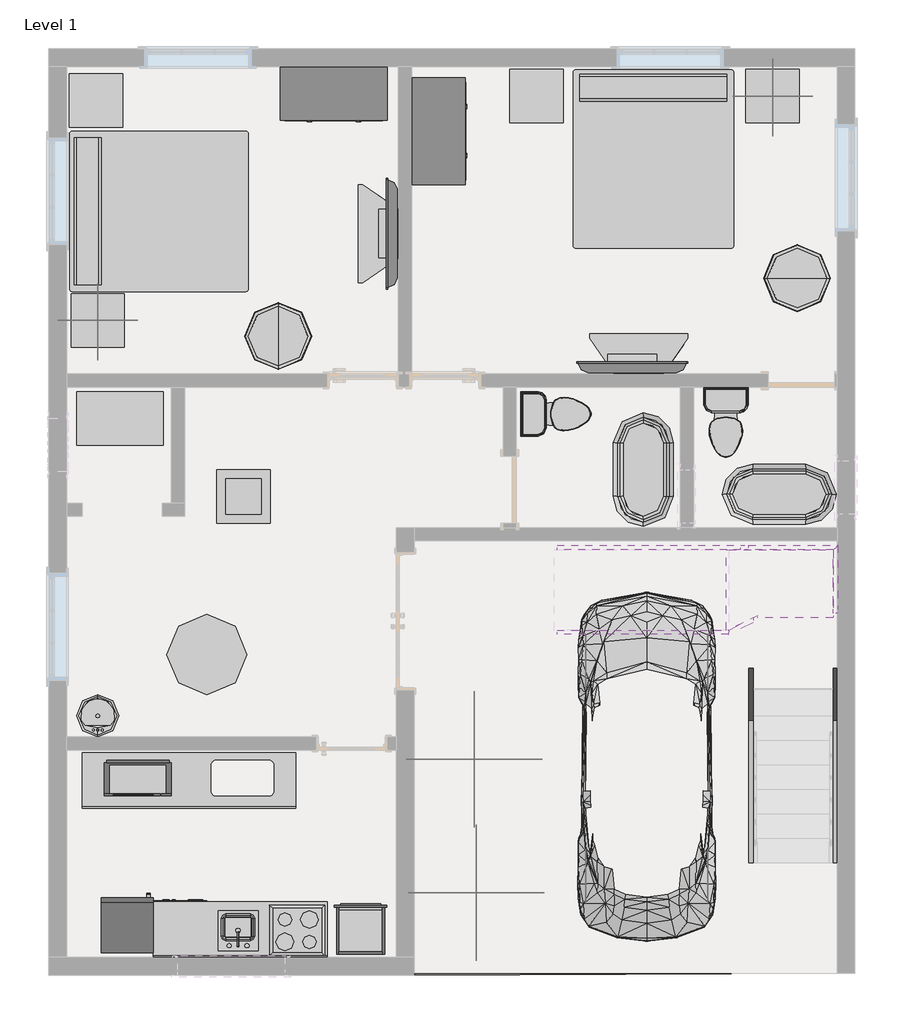
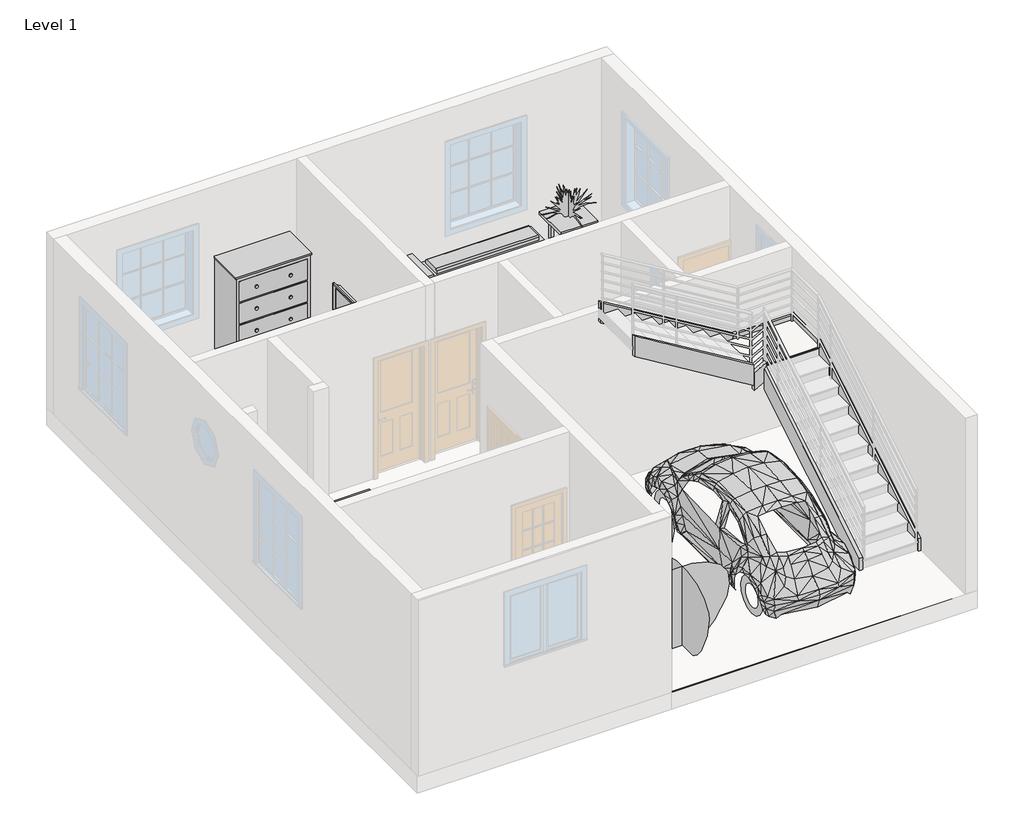
# One storey, part 5 of 5: 19 furniture elements, 8 proxies, 7 members, 6 flow terminals, 4 geographic elements, 1 slab.
"""IFC4 building model written with IfcOpenShell, lengths in millimetres."""

from ifc_helpers import new_model, si_unit, frame, origin, place, context, project, spatial, polyline, outline, extrude, faceted_brep, triangles, transform, mapped, element, save
from components import proxy_a6faaae8, proxy_45b28599, kitchenette_medium_kitchenette_medium_844211aa, proxy_8a8d5ab2, proxy_8b8c2dc4, rpc_beetle_rpc_beetle_3ce7ba48, proxy_c523a7b7, flow_terminal_871c2e40, flow_terminal_d49f872f, toilet_domestic_3d_toilet_domestic_3d_f7549cf7, toilet_domestic_3d_toilet_domestic_3d_183bbd19, flow_terminal_93af9e75, furniture_a8794613, furniture_22cae41e, furniture_c6510c7c, furniture_9fa109b2, furniture_fdf74506, tv_stand_tv_stand_6ce107e5, furniture_b5c51a22, furniture_905aceb5, furniture_5bc9ed15, furniture_d861f60e, furniture_ebfaaaa6, rpc_plant_tropical_agave_1_5_93a2a214, geographic_element_ca6e1e19, non_monolithic_landing_e53bceee

model = new_model("IFC4")

# Units and contexts
model_context = context("Model", 3, world=origin())
ifc_project = project(units=[si_unit("LENGTHUNIT", "METRE", prefix="MILLI")], contexts=[model_context])

# Site, building, storey
site = spatial("IfcSite", under=ifc_project)
building = spatial("IfcBuilding", under=site)
storey = spatial("IfcBuildingStorey", under=building, Name="Level 1", Elevation=0.0)

# Proxies
placement = place(None, origin())
element("IfcBuildingElementProxy", 1, Name="Building Element Proxy", at=placement, inside=storey, context=model_context, shape_type="Tessellation", body=[
    triangles([(-5848.5895203, 6522.5448944, 0.0), (-1156.9729843, 6792.048793, 0.0), (-1156.9729843, 2097.9200558, 0.0), (-5982.9731781, 2072.5200073, 0.0), (-5919.2578812, 6787.1200241, 0.0), (-5945.4754669, 6669.6818436, 0.0), (-5982.9731781, 7000.1198135, 0.0), (-1156.9729843, 6947.7020828, 0.0)], [[4, 6, 7], [5, 6, 1], [7, 5, 8], [5, 7, 6], [6, 4, 1], [1, 3, 2], [3, 1, 4], [2, 8, 1], [1, 8, 5]], closed=False),
])
proxy_shape = proxy_a6faaae8(model_context)
element("IfcBuildingElementProxy", 2, Name="Cook Top-4 Unit2 : 22\" x 20\"", ObjectType="Cook Top-4 Unit2 : 22\" x 20\"", at=placement, inside=storey, context=model_context, shape_type="MappedRepresentation", body=[
    mapped(proxy_shape, transform((-7316.4730118, 2580.5200123, 0.0), x_axis=(-1.0000000000000004, 0.0, 0.0), y_axis=(0.0, -1.0000000000000004, 0.0), z_axis=(0.0, 0.0, 1.0))),
])
proxy_2_shape = proxy_45b28599(model_context)
element("IfcBuildingElementProxy", 3, Name="Dishwasher : 24\" x 24\" x 34\"", ObjectType="Dishwasher : 24\" x 24\" x 34\"", at=placement, inside=storey, context=model_context, shape_type="MappedRepresentation", body=[
    mapped(proxy_2_shape, transform((-8267.6555433, 2872.3695771, 0.0), x_axis=(-1.0000000000000004, 0.0, 0.0), y_axis=(0.0, -1.0000000000000004, 0.0), z_axis=(0.0, 0.0, 1.0))),
])
kitchenette_medium_kitchenette_medium_shape = kitchenette_medium_kitchenette_medium_844211aa(model_context)
element("IfcBuildingElementProxy", 4, Name="Kitchenette - Medium : Kitchenette - Medium", ObjectType="Kitchenette - Medium : Kitchenette - Medium", at=placement, inside=storey, context=model_context, shape_type="MappedRepresentation", body=[
    mapped(kitchenette_medium_kitchenette_medium_shape, transform((-7640.6353069, 2275.7200123, 0.0), x_axis=(-1.0000000000000004, 0.0, 0.0), y_axis=(0.0, -1.0000000000000004, 0.0), z_axis=(0.0, 0.0, 1.0))),
])
proxy_3_shape = proxy_8a8d5ab2(model_context)
element("IfcBuildingElementProxy", 5, Name="Microwave : 30\" x 16\" x 18\"", ObjectType="Microwave : 30\" x 16\" x 18\"", at=placement, inside=storey, context=model_context, shape_type="MappedRepresentation", body=[
    mapped(proxy_3_shape, transform((-9632.8658891, 4673.5005181, 0.0), x_axis=(1.0000000000000007, 0.0, 0.0), y_axis=(0.0, 1.0000000000000007, 0.0), z_axis=(0.0, 0.0, 1.0))),
])
proxy_4_shape = proxy_8b8c2dc4(model_context)
element("IfcBuildingElementProxy", 6, Name="Oven Double-Built-in : 21 1/2\" x 39 1/4\" x 21\"", ObjectType="Oven Double-Built-in : 21 1/2\" x 39 1/4\" x 21\"", at=placement, inside=storey, context=model_context, shape_type="MappedRepresentation", body=[
    mapped(proxy_4_shape, transform((-6627.7479391, 2721.5858712, 0.0), x_axis=(-1.0000000000000004, 0.0, 0.0), y_axis=(0.0, -1.0000000000000004, 0.0), z_axis=(0.0, 0.0, 1.0))),
])
rpc_beetle_rpc_beetle_shape = rpc_beetle_rpc_beetle_3ce7ba48(model_context)
element("IfcBuildingElementProxy", 7, Name="RPC Beetle : RPC Beetle", ObjectType="RPC Beetle : RPC Beetle", at=placement, inside=storey, context=model_context, shape_type="MappedRepresentation", body=[
    mapped(rpc_beetle_rpc_beetle_shape, transform((-3328.6730118, 3215.5200123, 0.0), x_axis=(1.0, 0.0, 0.0), y_axis=(0.0, 1.0, 0.0), z_axis=(0.0, 0.0, 1.0))),
])
proxy_5_shape = proxy_c523a7b7(model_context)
element("IfcBuildingElementProxy", 8, Name="Refrigerator : 24\" x 25\" LH", ObjectType="Refrigerator : 24\" x 25\" LH", at=placement, inside=storey, context=model_context, shape_type="MappedRepresentation", body=[
    mapped(proxy_5_shape, transform((-9253.2230118, 2626.1689838, 0.0), x_axis=(-1.0000000000000004, 0.0, 0.0), y_axis=(0.0, -1.0000000000000004, 0.0), z_axis=(0.0, 0.0, 1.0))),
])

# Flow terminals
flow_terminal_shape = flow_terminal_871c2e40(model_context)
element("IfcFlowTerminal", 9, ObjectType="Sink Kitchen-Island : 18\" x 18\"", at=placement, inside=storey, context=model_context, shape_type="MappedRepresentation", body=[
    mapped(flow_terminal_shape, transform((-7973.8837712, 2582.8654134, -14.4), x_axis=(-1.0000000000000004, 0.0, 0.0), y_axis=(0.0, -1.0000000000000004, 0.0), z_axis=(0.0, 0.0, 1.0))),
])
flow_terminal_2_shape = flow_terminal_d49f872f(model_context)
element("IfcFlowTerminal", 10, ObjectType="Sink Vanity-Round : 19\" x 19\"", at=placement, inside=storey, context=model_context, shape_type="MappedRepresentation", body=[
    mapped(flow_terminal_2_shape, transform((-9493.1212712, 5116.6266447, 304.8), x_axis=(-1.0000000000000004, 0.0, 0.0), y_axis=(0.0, -1.0000000000000004, 0.0), z_axis=(0.0, 0.0, 1.0))),
])
toilet_domestic_3d_toilet_domestic_3d_shape = toilet_domestic_3d_toilet_domestic_3d_f7549cf7(model_context)
toilet_domestic_3d_toilet_domestic_3d_2_shape = toilet_domestic_3d_toilet_domestic_3d_183bbd19(model_context)
element("IfcFlowTerminal", 11, ObjectType="Toilet-Domestic-3D : Toilet-Domestic-3D", at=placement, inside=storey, context=model_context, shape_type="MappedRepresentation", body=[
    mapped(toilet_domestic_3d_toilet_domestic_3d_shape, transform((-2426.9730118, 8283.4239849, 0.0), x_axis=(1.0000000000000007, 0.0, 0.0), y_axis=(0.0, 1.0000000000000007, 0.0), z_axis=(0.0, 0.0, 1.0))),
    mapped(toilet_domestic_3d_toilet_domestic_3d_2_shape, transform((-2426.9730118, 8283.4239849, 0.0), x_axis=(1.0000000000000007, 0.0, 0.0), y_axis=(0.0, 1.0000000000000007, 0.0), z_axis=(0.0, 0.0, 1.0))),
])
element("IfcFlowTerminal", 12, ObjectType="Toilet-Domestic-3D : Toilet-Domestic-3D", at=placement, inside=storey, context=model_context, shape_type="MappedRepresentation", body=[
    mapped(toilet_domestic_3d_toilet_domestic_3d_shape, transform((-4269.0769845, 8473.3200123, 0.0), x_axis=(0.0, 1.0000000000000002, 0.0), y_axis=(-1.0000000000000002, 0.0, 0.0), z_axis=(0.0, 0.0, 1.0))),
    mapped(toilet_domestic_3d_toilet_domestic_3d_2_shape, transform((-4269.0769845, 8473.3200123, 0.0), x_axis=(0.0, 1.0000000000000002, 0.0), y_axis=(-1.0000000000000002, 0.0, 0.0), z_axis=(0.0, 0.0, 1.0))),
])
flow_terminal_3_shape = flow_terminal_93af9e75(model_context)
element("IfcFlowTerminal", 13, ObjectType="Tub-Free Standing-3D : 30\" x 60\"", at=placement, inside=storey, context=model_context, shape_type="MappedRepresentation", body=[
    mapped(flow_terminal_3_shape, transform((-1817.3730118, 7558.9200123, 0.0), x_axis=(0.0, -1.0000000000000002, 0.0), y_axis=(1.0000000000000002, 0.0, 0.0), z_axis=(0.0, 0.0, 1.0))),
])
element("IfcFlowTerminal", 14, ObjectType="Tub-Free Standing-3D : 30\" x 60\"", at=placement, inside=storey, context=model_context, shape_type="MappedRepresentation", body=[
    mapped(flow_terminal_3_shape, transform((-3366.7730118, 7838.3200123, 0.0), x_axis=(-1.0000000000000004, 0.0, 0.0), y_axis=(0.0, -1.0000000000000004, 0.0), z_axis=(0.0, 0.0, 1.0))),
])

# Furniture
furniture_shape = furniture_a8794613(model_context)
element("IfcFurniture", 15, ObjectType="Bed-Standard.0001 : King 78\" x 80\"", at=placement, inside=storey, context=model_context, shape_type="MappedRepresentation", body=[
    mapped(furniture_shape, transform((-8936.8680938, 10513.2314877, 0.0), x_axis=(0.0, 1.0000000000000002, 0.0), y_axis=(-1.0000000000000002, 0.0, 0.0), z_axis=(0.0, 0.0, 1.0))),
])
element("IfcFurniture", 16, ObjectType="Bed-Standard.0001 : King 78\" x 80\"", at=placement, inside=storey, context=model_context, shape_type="MappedRepresentation", body=[
    mapped(furniture_shape, transform((-3523.9615364, 11427.2150942, 0.0), x_axis=(1.0, 0.0, 0.0), y_axis=(0.0, 1.0, 0.0), z_axis=(0.0, 0.0, 1.0))),
])
furniture_2_shape = furniture_22cae41e(model_context)
element("IfcFurniture", 17, ObjectType="Counter Top w Sink Hole : 24\" Depth", at=placement, inside=storey, context=model_context, shape_type="MappedRepresentation", body=[
    mapped(furniture_2_shape, transform((-8529.6353069, 3977.5200123, 0.0), x_axis=(-1.0000000000000002, 0.0, 0.0), y_axis=(0.0, -1.0000000000000002, 0.0), z_axis=(0.0, 0.0, 1.0))),
])
furniture_3_shape = furniture_c6510c7c(model_context)
element("IfcFurniture", 18, ObjectType="Counter Top w Sink Hole : 24\" Depth", at=placement, inside=storey, context=model_context, shape_type="MappedRepresentation", body=[
    mapped(furniture_3_shape, transform((-8174.0353069, 2275.7200123, -14.4), x_axis=(-1.0000000000000004, 0.0, 0.0), y_axis=(0.0, -1.0000000000000004, 0.0), z_axis=(0.0, 0.0, 1.0))),
])
furniture_4_shape = furniture_9fa109b2(model_context)
element("IfcFurniture", 19, ObjectType="Dresser : 48\" x 72\" x 24\"", at=placement, inside=storey, context=model_context, shape_type="MappedRepresentation", body=[
    mapped(furniture_4_shape, transform((-6628.179752, 12494.0829664, 0.0), x_axis=(1.0, 0.0, 0.0), y_axis=(0.0, 1.0, 0.0), z_axis=(0.0, 0.0, 1.0))),
])
element("IfcFurniture", 20, ObjectType="Dresser : 48\" x 72\" x 24\"", at=placement, inside=storey, context=model_context, shape_type="MappedRepresentation", body=[
    mapped(furniture_4_shape, transform((-6066.7359659, 11968.3132721, 0.0), x_axis=(0.0, 1.0000000000000002, 0.0), y_axis=(-1.0000000000000002, 0.0, 0.0), z_axis=(0.0, 0.0, 1.0))),
])
furniture_5_shape = furniture_fdf74506(model_context)
element("IfcFurniture", 21, ObjectType="TV - Flat Screen : 50\"", at=placement, inside=storey, context=model_context, shape_type="MappedRepresentation", body=[
    mapped(furniture_5_shape, transform((-6232.0116355, 10526.7754981, 914.4), x_axis=(0.0, -1.0, 0.0), y_axis=(1.0, 0.0, 0.0), z_axis=(0.0, 0.0, 1.0))),
])
element("IfcFurniture", 22, ObjectType="TV - Flat Screen : 50\"", at=placement, inside=storey, context=model_context, shape_type="MappedRepresentation", body=[
    mapped(furniture_5_shape, transform((-3497.717526, 9001.7586359, 914.4), x_axis=(-1.0000000000000004, 0.0, 0.0), y_axis=(0.0, -1.0000000000000004, 0.0), z_axis=(0.0, 0.0, 1.0))),
])
tv_stand_tv_stand_shape = tv_stand_tv_stand_6ce107e5(model_context)
element("IfcFurniture", 23, ObjectType="TV Stand : TV Stand", at=placement, inside=storey, context=model_context, shape_type="MappedRepresentation", body=[
    mapped(tv_stand_tv_stand_shape, transform((-6160.7730118, 10655.9080143, 0.0), x_axis=(0.0, -1.0000000000000002, 0.0), y_axis=(1.0000000000000002, 0.0, 0.0), z_axis=(0.0, 0.0, 1.0))),
])
element("IfcFurniture", 24, ObjectType="TV Stand : TV Stand", at=placement, inside=storey, context=model_context, shape_type="MappedRepresentation", body=[
    mapped(tv_stand_tv_stand_shape, transform((-3292.3850097, 8930.5200123, 0.0), x_axis=(-1.0000000000000002, 0.0, 0.0), y_axis=(0.0, -1.0000000000000002, 0.0), z_axis=(0.0, 0.0, 1.0))),
])
furniture_6_shape = furniture_b5c51a22(model_context)
element("IfcFurniture", 25, ObjectType="Table-Coffee : 24\" x 24\" x 24\"", at=placement, inside=storey, context=model_context, shape_type="MappedRepresentation", body=[
    mapped(furniture_6_shape, transform((-7944.3387785, 7438.3089345, 0.0), x_axis=(1.0, 0.0, 0.0), y_axis=(0.0, 1.0, 0.0), z_axis=(0.0, 0.0, 1.0))),
])
furniture_7_shape = furniture_905aceb5(model_context)
element("IfcFurniture", 26, ObjectType="Table-Dining Round w Chairs : 36\" Diameter", at=placement, inside=storey, context=model_context, shape_type="MappedRepresentation", body=[
    mapped(furniture_7_shape, transform((-8448.854979, 5914.9987008, 0.0), x_axis=(1.0, 0.0, 0.0), y_axis=(0.0, 1.0, 0.0), z_axis=(0.0, 0.0, 1.0))),
])
furniture_8_shape = furniture_5bc9ed15(model_context)
element("IfcFurniture", 27, ObjectType="Table-Night Stand : 24\" x 24\" x 30\"", at=placement, inside=storey, context=model_context, shape_type="MappedRepresentation", body=[
    mapped(furniture_8_shape, transform((-9898.3066421, 9235.3200123, 0.0), x_axis=(1.0, 0.0, 0.0), y_axis=(0.0, 1.0, 0.0), z_axis=(0.0, 0.0, 1.0))),
])
element("IfcFurniture", 28, ObjectType="Table-Night Stand : 24\" x 24\" x 30\"", at=placement, inside=storey, context=model_context, shape_type="MappedRepresentation", body=[
    mapped(furniture_8_shape, transform((-9917.3566421, 11743.5700123, 0.0), x_axis=(1.0, 0.0, 0.0), y_axis=(0.0, 1.0, 0.0), z_axis=(0.0, 0.0, 1.0))),
])
element("IfcFurniture", 29, ObjectType="Table-Night Stand : 24\" x 24\" x 30\"", at=placement, inside=storey, context=model_context, shape_type="MappedRepresentation", body=[
    mapped(furniture_8_shape, transform((-2202.1066421, 11794.3700123, 0.0), x_axis=(1.0, 0.0, 0.0), y_axis=(0.0, 1.0, 0.0), z_axis=(0.0, 0.0, 1.0))),
])
element("IfcFurniture", 30, ObjectType="Table-Night Stand : 24\" x 24\" x 30\"", at=placement, inside=storey, context=model_context, shape_type="MappedRepresentation", body=[
    mapped(furniture_8_shape, transform((-4894.5066421, 11794.3700123, 0.0), x_axis=(1.0, 0.0, 0.0), y_axis=(0.0, 1.0, 0.0), z_axis=(0.0, 0.0, 1.0))),
])
furniture_9_shape = furniture_d861f60e(model_context)
element("IfcFurniture", 31, ObjectType="Table-Rectangular : 72\" x 30\"", at=placement, inside=storey, context=model_context, shape_type="MappedRepresentation", body=[
    mapped(furniture_9_shape, transform((-9335.7730118, 8422.5200123, 0.0), x_axis=(1.0, 0.0, 0.0), y_axis=(0.0, 1.0, 0.0), z_axis=(0.0, 0.0, 1.0))),
])
furniture_10_shape = furniture_ebfaaaa6(model_context)
element("IfcFurniture", 32, ObjectType="Table-Round : 36\" Diameter", at=placement, inside=storey, context=model_context, shape_type="MappedRepresentation", body=[
    mapped(furniture_10_shape, transform((-7532.3730118, 9362.3200123, 0.0), x_axis=(0.0, 1.0000000000000002, 0.0), y_axis=(-1.0000000000000002, 0.0, 0.0), z_axis=(0.0, 0.0, 1.0))),
])
element("IfcFurniture", 33, ObjectType="Table-Round : 36\" Diameter", at=placement, inside=storey, context=model_context, shape_type="MappedRepresentation", body=[
    mapped(furniture_10_shape, transform((-1614.1730118, 10022.7200123, 0.0), x_axis=(1.0, 0.0, 0.0), y_axis=(0.0, 1.0, 0.0), z_axis=(0.0, 0.0, 1.0))),
])

# Geographic elements
rpc_plant_tropical_agave_1_5_shape = rpc_plant_tropical_agave_1_5_93a2a214(model_context)
element("IfcGeographicElement", 34, ObjectType="RPC Plant - Tropical : Agave - 1.5'", at=placement, inside=storey, context=model_context, shape_type="MappedRepresentation", body=[
    mapped(rpc_plant_tropical_agave_1_5_shape, transform((-9589.7730118, 9540.1200123, 762.0), x_axis=(1.0, 0.0, 0.0), y_axis=(0.0, 1.0, 0.0), z_axis=(0.0, 0.0, 1.0))),
])
element("IfcGeographicElement", 35, ObjectType="RPC Plant - Tropical : Agave - 1.5'", at=placement, inside=storey, context=model_context, shape_type="MappedRepresentation", body=[
    mapped(rpc_plant_tropical_agave_1_5_shape, transform((-1893.5730118, 12099.1700123, 762.0), x_axis=(1.0, 0.0, 0.0), y_axis=(0.0, 1.0, 0.0), z_axis=(0.0, 0.0, 1.0))),
])
geographic_element_shape = geographic_element_ca6e1e19(model_context)
element("IfcGeographicElement", 36, ObjectType="RPC Shrub : Burning Bush 4'-6\"", at=placement, inside=storey, context=model_context, shape_type="MappedRepresentation", body=[
    mapped(geographic_element_shape, transform((-5271.7730118, 3012.3200123, 0.0), x_axis=(1.0, 0.0, 0.0), y_axis=(0.0, 1.0, 0.0), z_axis=(0.0, 0.0, 1.0))),
])
element("IfcGeographicElement", 37, ObjectType="RPC Shrub : Burning Bush 4'-6\"", at=placement, inside=storey, context=model_context, shape_type="MappedRepresentation", body=[
    mapped(geographic_element_shape, transform((-5297.1730118, 4536.3200123, 0.0), x_axis=(1.0, 0.0, 0.0), y_axis=(0.0, 1.0, 0.0), z_axis=(0.0, 0.0, 1.0))),
])

# Members
element("IfcMember", 38, ObjectType="Stringer - 2\" Width", at=placement, inside=storey, context=model_context, shape_type="Brep", body=[
    faceted_brep([(-2115.3932736, 3353.09939, 0.0), (-2166.1932736, 3353.09939, 0.0), (-2166.1932736, 3591.1849018, 0.0), (-2115.3932736, 3591.1849018, 0.0), (-2115.3932736, 3353.09939, 212.114512), (-2166.1932736, 3353.09939, 212.114512), (-2115.3932736, 6090.4746443, 1871.1298176), (-2166.1932736, 6065.460212, 1855.9695556), (-2166.1932736, 6065.460212, 1499.5607941), (-2115.3932736, 6090.4746443, 1514.7210561)], [[[0, 1, 2, 3]], [[4, 5, 1, 0]], [[5, 4, 6, 7]], [[1, 5, 7, 8, 2]], [[4, 0, 3, 9, 6]], [[2, 8, 9, 3]], [[6, 9, 8, 7]]]),
])
element("IfcMember", 39, ObjectType="Stringer - 2\" Width", at=placement, inside=storey, context=model_context, shape_type="SweptSolid", body=[
    extrude(outline(polyline([(3353.09939, 0.0), (3353.09939, 212.114512), (6202.2404453, 1938.8666667), (6287.3949018, 1634.0666667), (3591.1849018, 0.0), (3353.09939, 0.0)])), frame((-1200.9932736, 0.0, 0.0), z_axis=(1.0, 0.0, 0.0), x_axis=(0.0, 1.0, 0.0)), (0.0, 0.0, 1.0), 50.8),
])
element("IfcMember", 40, ObjectType="Stringer - 2\" Width", at=placement, inside=storey, context=model_context, shape_type="SweptSolid", body=[
    extrude(outline(polyline([(1718.3724171, -2394.7932736), (2074.7811786, -2394.7932736), (3260.114512, -4350.5932736), (2903.7057504, -4350.5932736), (1718.3724171, -2394.7932736)])), frame((0.0, 5958.7200123, 0.0), z_axis=(0.0, 1.0, 0.0), x_axis=(0.0, 0.0, 1.0)), (0.0, 0.0, 1.0), 50.8),
])
element("IfcMember", 41, ObjectType="Stringer - 2\" Width", at=placement, inside=storey, context=model_context, shape_type="SweptSolid", body=[
    extrude(outline(polyline([(1634.0666667, -2255.6887853), (1938.8666667, -2170.5343288), (3260.114512, -4350.5932736), (2903.7057504, -4350.5932736), (1634.0666667, -2255.6887853)])), frame((0.0, 6923.9200123, 0.0), z_axis=(0.0, 1.0, 0.0), x_axis=(0.0, 0.0, 1.0)), (0.0, 0.0, 1.0), 50.8),
])
element("IfcMember", 42, ObjectType="Stringer - 2\" Width", at=placement, inside=storey, context=model_context, shape_type="SweptSolid", body=[
    extrude(outline(polyline([(-2394.7932736, 5952.8952666), (-2394.7932736, 6009.5200123), (-2115.3932736, 6147.09939), (-2115.3932736, 6090.4746443), (-2394.7932736, 5952.8952666)])), frame((0.0, 0.0, 1634.0666667), z_axis=(0.0, 0.0, 1.0), x_axis=(1.0, 0.0, 0.0)), (0.0, 0.0, 1.0), 304.8),
])
element("IfcMember", 43, ObjectType="Stringer - 2\" Width", at=placement, inside=storey, context=model_context, shape_type="Brep", body=[
    faceted_brep([(-1200.9932736, 6202.2404453, 1938.8666667), (-1150.1932736, 6202.2404453, 1938.8666667), (-1150.1932736, 6974.7200123, 1938.8666667), (-1200.9932736, 6923.9200123, 1938.8666667), (-1200.9932736, 6287.3949018, 1634.0666667), (-1200.9932736, 6923.9200123, 1634.0666667), (-1150.1932736, 6287.3949018, 1634.0666667), (-1150.1932736, 6974.7200123, 1634.0666667)], [[[0, 1, 2, 3]], [[4, 0, 3, 5]], [[6, 4, 5, 7]], [[1, 6, 7, 2]], [[1, 0, 4, 6]], [[2, 7, 5, 3]]]),
])
element("IfcMember", 44, ObjectType="Stringer - 2\" Width", at=placement, inside=storey, context=model_context, shape_type="Brep", body=[
    faceted_brep([(-1200.9932736, 6923.9200123, 1938.8666667), (-1150.1932736, 6974.7200123, 1938.8666667), (-2170.5343288, 6974.7200123, 1938.8666667), (-2170.5343288, 6923.9200123, 1938.8666667), (-1200.9932736, 6923.9200123, 1634.0666667), (-2255.6887853, 6923.9200123, 1634.0666667), (-1150.1932736, 6974.7200123, 1634.0666667), (-2255.6887853, 6974.7200123, 1634.0666667)], [[[0, 1, 2, 3]], [[4, 0, 3, 5]], [[6, 4, 5, 7]], [[1, 6, 7, 2]], [[1, 0, 4, 6]], [[2, 7, 5, 3]]]),
])

# Slab
non_monolithic_landing_shape = non_monolithic_landing_e53bceee(model_context)
element("IfcSlab", 45, ObjectType="Non-Monolithic Landing", at=placement, inside=storey, context=model_context, shape_type="MappedRepresentation", body=[
    mapped(non_monolithic_landing_shape, transform((0.0, 0.0, 0.0), x_axis=(1.0, 0.0, 0.0), y_axis=(0.0, 1.0, 0.0), z_axis=(0.0, 0.0, 1.0))),
])

save(model, "model.ifc")

# Revit data of these elements
# Type "Cook Top-4 Unit2 : 22\" x 20\""
#   Depth = 1' - 8"
#   Width = 1' - 10"
#   Burner Material = Steel, Chrome Plated
#   Cooktop Material = Steel, Polished
#   Default Elevation = 0
#   Assembly Code = ""
# Type "Dishwasher : 24\" x 24\" x 34\""
#   Label = "DW"
#   Assembly Code = "E1090400"
#   Depth = 2' - 0"
#   Height = 2' - 10"
#   Width = 2' - 0"
#   Dishwasher Material = Steel, Paint Finish, Ivory, Glossy
#   Panel Face Material = Plastic, Opaque Black
#   Default Elevation = 0
# Type "Kitchenette - Medium : Kitchenette - Medium"
#   Assembly Code = "E1090400"
#   Counter Length = 6' - 6"
#   Cabinet Width = 4' - 6"
#   Cabinet Height = 2' - 10 1/2"
#   Cabinet Depth = 2' - 0"
#   Toe Depth = 0' - 3"
#   Toe Height = 0' - 3 1/2"
#   Cabinet Material = Cabinets
#   Door/Drawer Material = Cabinets
#   Handle Material = Cabinets - Handles
#   Default Elevation = 0
# Type "Microwave : 30\" x 16\" x 18\""
#   Assembly Code = "E1090400"
#   Depth = 1' - 4"
#   Height = 1' - 6"
#   Width = 2' - 6"
#   Microwave Material = Laminate, Ivory, Matte
#   Default Elevation = 0
# Type "Oven Double-Built-in : 21 1/2\" x 39 1/4\" x 21\""
#   Label = "OVEN"
#   Assembly Code = "E1090400"
#   Depth = 1' - 9"
#   Height = 3' - 3 1/4"
#   Width = 1' - 9 1/2"
#   Oven Material = Metal - Stainless Steel, Polished
#   Default Elevation = 0
# Type "RPC Beetle : RPC Beetle"
#   built-in parameter 1005195 = "RPC-16-0U6E-L4EG-ENH1-J3KF-SVEL-0TX4-C0"
#   Height = 0
# Type "Refrigerator : 24\" x 25\" LH"
#   Label = "REF."
#   Assembly Code = "E1090400"
#   Depth = 2' - 0 3/4"
#   Handle = 0' - 1 1/2"
#   Height = 5' - 3 1/2"
#   Rear Clearance = 0' - 2"
#   Top Door Height = 1' - 8"
#   Width = 1' - 11 1/2"
#   Material = Steel, Paint Finish, Ivory, Glossy
#   Default Elevation = 0
# Type "Sink Kitchen-Island : 18\" x 18\""
#   Assembly Code = "D2010410"
#   Counter Height = 3' - 0"
#   Depth = 1' - 6"
#   Width = 1' - 6"
#   Faucet Material = Steel, Polished
#   Sink Material = Steel, Polished
#   Default Elevation = 0
# Type "Sink Vanity-Round : 19\" x 19\""
#   Assembly Code = "D2010400"
#   Top Of Counter = 2' - 7"
#   Basin Material = Porcelain, Linen
#   Faucet Material = Steel, Polished
#   Default Elevation = 0
# Type "Toilet-Domestic-3D : Toilet-Domestic-3D"
#   Assembly Code = "D2010110"
#   Toilet - Bowl/Basin Material = Porcelain, Linen
#   Toilet - Seat Material = Laminate, Linen, Matte
#   Default Elevation = 0
# Type "Tub-Free Standing-3D : 30\" x 60\""
#   Assembly Code = "D2010110"
#   Height = 1' - 6"
#   Length = 4' - 3"
#   Width = 2' - 3"
#   Tub Material = Porcelain, Ivory
#   Default Elevation = 0
# Type "Bed-Standard.0001 : King 78\" x 80\""
#   Assembly Code = "E2020200"
#   Length = 6' - 8"
#   Width = 6' - 0"
#   Leg Material = Steel, Chrome Plated
#   Mattress Material = Linen, White
#   Default Elevation = 0
# Type "Counter Top w Sink Hole : 24\" Depth"
#   Assembly Code = "C1030400"
#   Counter Thickness = 0' - 1 1/2"
#   Depth = 2' - 1"
#   Height = 3' - 0"
#   Length [instance default] = 8' - 0"
#   Sink Location [instance default] = 2' - 0"
#   Sink Location To Wall [instance default] = 0' - 6"
#   Sink Opening Depth [instance default] = 1' - 3"
#   Sink Opening Width [instance default] = 2' - 3"
#   Counter Top Material = none
#   Default Elevation = 0
# Type "Dresser : 48\" x 72\" x 24\""
#   Assembly Code = "E2020200"
#   Depth = 2' - 0"
#   Height = 6' - 0"
#   Width = 4' - 0"
#   Dresser Material = Laminate - Ivory, Glossy
#   Drawer Material = Laminate, Ivory, Matte
#   Knob Material = Cherry
#   Default Elevation = 0
# Type "TV - Flat Screen : 50\""
#   SinAng = 0' - 0.0193"
#   L = 3' - 7.57782"
#   H = 2' - 0.51477"
#   Thickness = 0' - 4.33071"
#   Diagonal = 4' - 2"
#   CosAng = 0' - 0.03431"
#   Stand [instance default] = yes
#   Default Elevation = 0
# Type "TV Stand : TV Stand"
#   Depth = 1' - 6"
#   Width = 3' - 8"
#   Height = 1' - 7 1/2"
#   Finish = Melamine - Gray
#   Default Elevation = 0
# Type "Table-Coffee : 24\" x 24\" x 24\""
#   Assembly Code = "E2020200"
#   Height = 2' - 0"
#   Length = 2' - 0"
#   Width = 2' - 0"
#   Top Material = none
#   Frame Material = none
#   Default Elevation = 0
# Type "Table-Dining Round w Chairs : 36\" Diameter"
#   Assembly Code = "E2020200"
#   Radius = 1' - 6"
#   Diameter = 3' - 0"
#   Height = 2' - 6"
#   Chairs = 4
#   Base Material = Pine
#   Top Material = Laminate, Linen, Matte
#   Default Elevation = 0
# Type "Table-Night Stand : 24\" x 24\" x 30\""
#   Assembly Code = "E2020200"
#   Depth = 2' - 0"
#   Height = 2' - 6"
#   Width = 2' - 0"
#   Base Material = Birch
#   Top Material = Laminate, Ivory, Matte
#   Default Elevation = 0
# Type "Table-Rectangular : 72\" x 30\""
#   Assembly Code = "E2020200"
#   Height = 2' - 6"
#   Length = 3' - 3"
#   Width = 2' - 0"
#   Base Material = Birch
#   Top Material = Birch
#   Default Elevation = 0
# Type "Table-Round : 36\" Diameter"
#   Assembly Code = "E2020200"
#   Base Radius = 0' - 10"
#   Height = 2' - 6"
#   Radius = 1' - 3"
#   Base Material = Steel, Chrome Plated
#   Top Material = Birch
#   Default Elevation = 0
# Type "RPC Plant - Tropical : Agave - 1.5'"
#   built-in parameter 1005198 = "{2, 15},{39, RPC-16-G1GJ-63FX-7K5P-N000-ST1L-LVER-AU},{1, 0},{1, 0},{2, 13},{1, 8},{5, Color},{1, 0},{1, 0},{3, 0.8},{3, 0.8},{3, 0.8},{1, 8},{7, BBoxMin},{1, 0},{1, 0},{1, 0},{1, 0},{1, 0},{1, 8},{7, BBoxMax},{1, 0},{1, 0},{1, 0},{1, 0},{1, 0},{2, 11},{9, RPCTypeId},{1, 0},{1, 0},{39, RPC-16-G1GJ-63FX-7K5P-N000-ST1L-LVER-AU},{1, 6},{14, RPCPlantHeight},{1, 0},{1, 0},{3, 1.5},{2, 11},{7, keyword},{1, 0},{1, 0},{35, :RPCs:Plants [General]:Geometry:RPC},{2, 11},{8, category},{1, 0},{1, 0},{16, Plants [General]},{2, 11},{12, LocalizedUID},{1, 0},{1, 0},{5, Agave},{2, 14},{6, Height},{1, 0},{1, 0},{3, 1.5},{1, 2},{16, Cast Reflections},{1, 0},{1, 0},{1, 0},{1, 2},{12, Cast Shadows},{1, 0},{1, 0},{1, 1},{1, 2},{9, Lock View},{1, 0},{1, 0},{1, 0},{1, 4},{5, ViewC},{1, 0},{1, 0},{1, 0},{21, assetlibrary_base.fbx},{1, 5},"
#   built-in parameter 1005195 = "RPC-16-G1GJ-63FX-7K5P-N000-ST1L-LVER-AU"
#   Type Comments = "Agave"
#   Assembly Code = "G2050500"
#   Height = 1' - 6"
#   Default Elevation = 0
# Type "RPC Shrub : Burning Bush 4'-6\""
#   Type Comments = "Burning Bush"
#   built-in parameter 1005198 = "{2, 15},{39, RPC-16-FVGW-0UXX-7JA7-N000-ST1L-LVER-AU},{1, 0},{1, 0},{2, 13},{1, 8},{5, Color},{1, 0},{1, 0},{3, 0.8},{3, 0.8},{3, 0.8},{1, 8},{7, BBoxMin},{1, 0},{1, 0},{1, 0},{1, 0},{1, 0},{1, 8},{7, BBoxMax},{1, 0},{1, 0},{1, 0},{1, 0},{1, 0},{2, 11},{9, RPCTypeId},{1, 0},{1, 0},{39, RPC-16-FVGW-0UXX-7JA7-N000-ST1L-LVER-AU},{1, 6},{14, RPCPlantHeight},{1, 0},{1, 0},{3, 4.5},{2, 11},{7, keyword},{1, 0},{1, 0},{35, :RPCs:Shrubs & Grasses:Geometry:RPC},{2, 11},{8, category},{1, 0},{1, 0},{16, Shrubs & Grasses},{2, 11},{12, LocalizedUID},{1, 0},{1, 0},{12, Burning Bush},{2, 14},{6, Height},{1, 0},{1, 0},{3, 4.5},{1, 2},{16, Cast Reflections},{1, 0},{1, 0},{1, 0},{1, 2},{12, Cast Shadows},{1, 0},{1, 0},{1, 1},{1, 2},{9, Lock View},{1, 0},{1, 0},{1, 0},{1, 4},{5, ViewC},{1, 0},{1, 0},{1, 0},{21, assetlibrary_base.fbx},{1, 5},"
#   built-in parameter 1005195 = "RPC-16-FVGW-0UXX-7JA7-N000-ST1L-LVER-AU"
#   Assembly Code = "G2050500"
#   Height = 4' - 6"
#   Default Elevation = 0
# Element 1 (IfcBuildingElementProxy)
#   Material = none
#   Phase Created = New Construction
# Element 2 (IfcBuildingElementProxy, "Cook Top-4 Unit2 : 22\" x 20\"")
#   Phase Created = New Construction
#   Materials on its faces: "Steel, Chrome Plated", "Steel, Polished"
# Element 3 (IfcBuildingElementProxy, "Dishwasher : 24\" x 24\" x 34\"")
#   Phase Created = New Construction
#   Materials on its faces: "Steel, Paint Finish, Ivory, Glossy", "Plastic, Opaque Black"
# Element 4 (IfcBuildingElementProxy, "Kitchenette - Medium : Kitchenette - Medium")
#   Phase Created = New Construction
#   Materials on its faces: "Cabinets", "Cabinets - Handles"
# Element 5 (IfcBuildingElementProxy, "Microwave : 30\" x 16\" x 18\"")
#   Phase Created = New Construction
#   Materials on its faces: "Laminate, Ivory, Matte", "Glass"
# Element 6 (IfcBuildingElementProxy, "Oven Double-Built-in : 21 1/2\" x 39 1/4\" x 21\"")
#   Phase Created = New Construction
#   Materials on its faces: "Steel", "Metal - Stainless Steel, Polished", "Glass"
# Element 7 (IfcBuildingElementProxy, "RPC Beetle : RPC Beetle")
#   Phase Created = New Construction
# Element 8 (IfcBuildingElementProxy, "Refrigerator : 24\" x 25\" LH")
#   Phase Created = New Construction
#   Materials on its faces: "Steel, Paint Finish, Ivory, Glossy", "Steel, Chrome Plated"
# Element 9 (IfcFlowTerminal, "Sink Kitchen-Island : 18\" x 18\"")
#   Mark = "5"
#   Phase Created = New Construction
#   Materials on its faces: "Steel, Polished"
# Element 10 (IfcFlowTerminal, "Sink Vanity-Round : 19\" x 19\"")
#   Mark = "6"
#   Phase Created = New Construction
#   Materials on its faces: "Porcelain, Linen", "Steel, Polished"
# Element 11 (IfcFlowTerminal, "Toilet-Domestic-3D : Toilet-Domestic-3D")
#   Mark = "1"
#   Phase Created = New Construction
#   Materials on its faces: "Porcelain, Linen", "Laminate, Linen, Matte"
# Element 12 (IfcFlowTerminal, "Toilet-Domestic-3D : Toilet-Domestic-3D")
#   Mark = "2"
#   Phase Created = New Construction
#   Materials on its faces: "Porcelain, Linen", "Laminate, Linen, Matte"
# Element 13 (IfcFlowTerminal, "Tub-Free Standing-3D : 30\" x 60\"")
#   Mark = "3"
#   Phase Created = New Construction
#   Materials on its faces: "Porcelain, Ivory"
# Element 14 (IfcFlowTerminal, "Tub-Free Standing-3D : 30\" x 60\"")
#   Mark = "4"
#   Phase Created = New Construction
#   Materials on its faces: "Porcelain, Ivory"
# Elements 15, 16 (IfcFurniture, "Bed-Standard.0001 : King 78\" x 80\"")
#   Phase Created = New Construction
#   Materials on its faces: "Linen, White", "Steel, Chrome Plated"
# Element 17 (IfcFurniture, "Counter Top w Sink Hole : 24\" Depth")
#   Sink Opening Width = 2' - 3"
#   Sink Opening Depth = 1' - 3"
#   Sink Location To Wall = 0' - 6"
#   Sink Location = 2' - 0"
#   Length = 8' - 0"
#   Phase Created = New Construction
#   Materials on its faces: "Counter Top"
# Element 18 (IfcFurniture, "Counter Top w Sink Hole : 24\" Depth")
#   Sink Opening Depth = 1' - 2"
#   Sink Location To Wall = 0' - 6"
#   Length = 6' - 6"
#   Sink Location = 3' - 4"
#   Sink Opening Width = 1' - 4"
#   Phase Created = New Construction
#   Materials on its faces: "Counter Top"
# Elements 19, 20 (IfcFurniture, "Dresser : 48\" x 72\" x 24\"")
#   Phase Created = New Construction
#   Materials on its faces: "Laminate, Ivory, Matte", "Cherry", "Laminate - Ivory, Glossy"
# Elements 21, 22 (IfcFurniture, "TV - Flat Screen : 50\"")
#   Stand = yes
#   Phase Created = New Construction
#   Materials on its faces: "TV - Black", "TV - Glass", "TV - Screen"
# Elements 23, 24 (IfcFurniture, "TV Stand : TV Stand")
#   Phase Created = New Construction
#   Materials on its faces: "Melamine - Gray", "Glass - Shelves"
# Element 25 (IfcFurniture, "Table-Coffee : 24\" x 24\" x 24\"")
#   Phase Created = New Construction
#   Materials on its faces: "Glass - Clear, Grey"
# Element 26 (IfcFurniture, "Table-Dining Round w Chairs : 36\" Diameter")
#   Phase Created = New Construction
#   Materials on its faces: "Pine", "Laminate, Linen, Matte"
# Elements 27, 28, 29, 30 (IfcFurniture, "Table-Night Stand : 24\" x 24\" x 30\"")
#   Phase Created = New Construction
#   Materials on its faces: "Birch", "Laminate, Ivory, Matte"
# Element 31 (IfcFurniture, "Table-Rectangular : 72\" x 30\"")
#   Phase Created = New Construction
#   Materials on its faces: "Birch"
# Elements 32, 33 (IfcFurniture, "Table-Round : 36\" Diameter")
#   Phase Created = New Construction
#   Materials on its faces: "Steel, Chrome Plated", "Birch"
# Elements 34, 35 (IfcGeographicElement, "RPC Plant - Tropical : Agave - 1.5'")
#   Phase Created = New Construction
# Elements 36, 37 (IfcGeographicElement, "RPC Shrub : Burning Bush 4'-6\"")
#   Phase Created = New Construction
# Elements 38, 39, 40, 41, 42, 43, 44 (IfcMember, "Stringer - 2\" Width")
#   Phase Created = New Construction
# Element 45 (IfcSlab, "Non-Monolithic Landing")
#   Phase Created = New Construction
# Materials
#   "Steel, Chrome Plated": class "Metal", colour RGB 17 17 17, transparency 0, Description = "Chromiuim plated steel", Cost = 0
#   "Steel, Polished": class "Metal", colour RGB 57 57 57, transparency 0, Description = "Polished steel", Cost = 0
#   "Steel, Paint Finish, Ivory, Glossy": class "Metal", colour RGB 247 247 239, transparency 0, Description = "Steel, paint finish, ivory, glossy", Cost = 0
#   "Plastic, Opaque Black": class "Plastic", colour RGB 0 0 0, transparency 0.7, Description = "Plastic, generic, opaque black", Cost = 0
#   "Cabinets": colour RGB 249 249 249, transparency 0
#   "Cabinets - Handles": class "Metal", colour RGB 57 57 57, transparency 0
#   "Laminate, Ivory, Matte": class "Plastic", colour RGB 247 247 239, transparency 0, Description = "Plastic Laminate - Ivory, Matte", Cost = 0
#   "Metal - Stainless Steel, Polished": class "Metal", colour RGB 216 216 216, transparency 0
#   "Porcelain, Linen": class "Ceramic", colour RGB 249 239 230, transparency 0, Description = "Porcelain, linen", Cost = 0
#   "Laminate, Linen, Matte": class "Plastic", colour RGB 249 239 230, transparency 0, Description = "Plastic Laminate - Linen, Matte", Cost = 0
#   "Porcelain, Ivory": class "Ceramic", colour RGB 247 247 239, transparency 0, Description = "Porcelain, ivory", Cost = 0
#   "Linen, White": class "Textile", colour RGB 247 247 239, transparency 0, Description = "Linen, white", Cost = 0
#   "Laminate - Ivory, Glossy": colour RGB 247 247 239, transparency 0
#   "Cherry": class "Wood", colour RGB 226 177 128, transparency 0, Description = "Prunus Serotina", Cost = 0
#   "Melamine - Gray": class "Wood", colour RGB 49 49 49, transparency 0
#   "Pine": class "Wood", colour RGB 223 192 134, transparency 0, Description = "Pinus Echinata", Cost = 0
#   "Birch": class "Wood", colour RGB 224 178 126, transparency 0, Description = "Betula Alleghaniensis", Cost = 0
#   "Glass": class "Glass", colour RGB 0 128 192, transparency 0.75, Description = "Soda Lime Glass", Cost = 0
#   "Steel": class "Metal", colour RGB 247 247 247, transparency 0, Description = "Steel, mill finish", Cost = 0
#   "Counter Top": class "Wood", colour RGB 226 177 128, transparency 0
#   "TV - Black": colour RGB 49 49 49, transparency 0
#   "TV - Glass": colour RGB 157 157 157, transparency 0.9
#   "TV - Screen": colour RGB 0 0 0, transparency 0
#   "Glass - Shelves": class "Glass", colour RGB 167 167 167, transparency 0.9
#   "Glass - Clear, Grey": class "Glass", colour RGB 252 255 255, transparency 0.64
